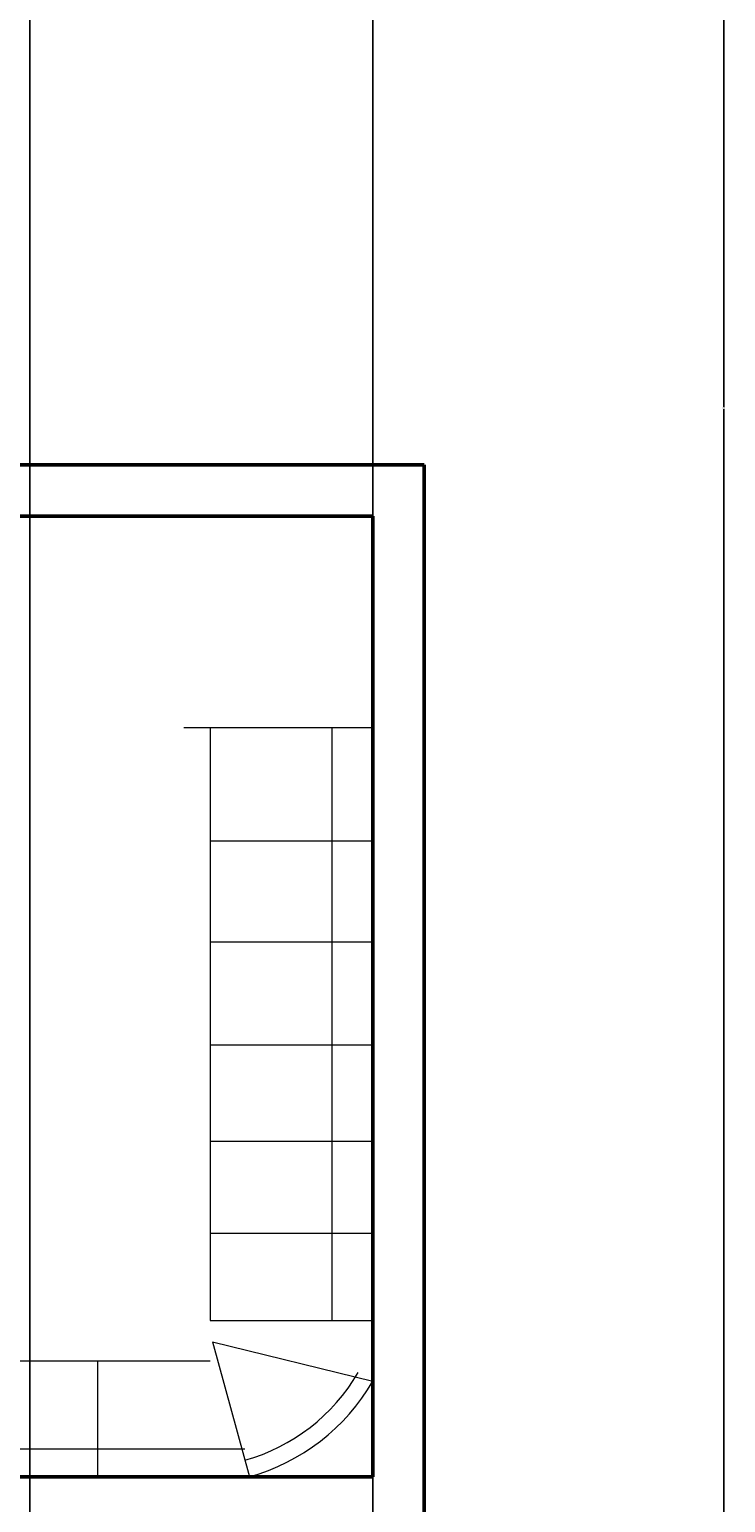
# Model space of a CAD drawing. Units: inches. Extents: x 5375 to 6084, y 16106 to 17259.
# Tile 26 of 32: x 5963 to 6084, y 16518 to 16776. Entities that reach past the tile are written whole.
import ezdxf

# ---------------------------------------------------------------- set-up
doc = ezdxf.new("R2010")
doc.units = ezdxf.units.IN
for name, color, linetype, lineweight in [('A-ANNO-DIMS', 2, 'Continuous', 18), ('FURNITURE', 3, 'Continuous', 18), ('WALL', 6, 'Continuous', 50)]:
    doc.layers.add(name, color=color, linetype=linetype, lineweight=lineweight)
doc.styles.get("Standard").update_dxf_attribs({"font": 'arial.ttf'})
doc.dimstyles.get("Standard").update_dxf_attribs({"dimtxt": 0.18, "dimasz": 0.18, "dimexe": 0.18, "dimexo": 0.0625, "dimgap": 0.09, "dimtad": 0, "dimtih": 1, "dimtoh": 1, "dimdec": 4, "dimzin": 0, "dimdsep": 46, "dimtxsty": 'Standard', "dimcen": 0.09, "dimadec": 0, "dimazin": 0, "dimtfac": 1, "dimtdec": 4, "dimtofl": 0, "dimtmove": 0, "dimatfit": 3, "dimfxl": 1, "dimtolj": 1, "dimtzin": 0, "dimarcsym": 0})

# ---------------------------------------------------------------- blocks, each defined once
blk = doc.blocks.new('*D31')
at = {"layer": 'A-ANNO-DIMS', "color": 0, "lineweight": -2, "transparency": 16777216}
for p, q in [((6031.68, 17206.58), (6084.2, 17206.58)), ((6084.02, 17206.4), (6084.02, 16709.66)), ((6084.02, 16212.56), (6084.02, 16709.3)), ((6031.68, 16212.38), (6084.2, 16212.38))]:
    blk.add_line(p, q, dxfattribs=at)
at = {"layer": 'A-ANNO-DIMS', "color": 0, "transparency": 16777216}
for points in [[(6083.99, 17206.4), (6084.05, 17206.4), (6084.02, 17206.58)], [(6083.99, 16212.56), (6084.05, 16212.56), (6084.02, 16212.38)]]:
    blk.add_solid(points, dxfattribs=at)
at = {"layer": 'Defpoints', "color": 0, "transparency": 16777216}
for p in [(6031.62, 17206.58), (6084.02, 17206.58), (6031.62, 16212.38)]:
    blk.add_point(p, dxfattribs=at)
at = {"layer": 'A-ANNO-DIMS', "color": 0, "transparency": 16777216, "insert": (6084.02, 16709.48), "char_height": 0.18, "attachment_point": 5}
blk.add_mtext('\\A1;994.2', dxfattribs=at)
blk = doc.blocks.new('*D48')
at = {"layer": 'A-ANNO-DIMS', "color": 0, "lineweight": -2, "transparency": 16777216}
for p, q in [((5962.62, 16411.64), (5962.62, 17259.16)), ((5962.8, 17258.98), (5992.4, 17258.98)), ((6022.44, 17258.98), (5992.84, 17258.98)), ((6022.62, 16411.64), (6022.62, 17259.16))]:
    blk.add_line(p, q, dxfattribs=at)
at = {"layer": 'A-ANNO-DIMS', "color": 0, "transparency": 16777216}
for points in [[(5962.8, 17259.01), (5962.8, 17258.95), (5962.62, 17258.98)], [(6022.44, 17259.01), (6022.44, 17258.95), (6022.62, 17258.98)]]:
    blk.add_solid(points, dxfattribs=at)
at = {"layer": 'Defpoints', "color": 0, "transparency": 16777216}
for p in [(6022.62, 17258.98), (5962.62, 16411.58), (6022.62, 16411.58)]:
    blk.add_point(p, dxfattribs=at)
at = {"layer": 'A-ANNO-DIMS', "color": 0, "transparency": 16777216, "insert": (5992.62, 17258.98), "char_height": 0.18, "attachment_point": 5}
blk.add_mtext('\\A1;60', dxfattribs=at)

msp = doc.modelspace()

# ---------------------------------------------------------------- linework, layer by layer
at = {"layer": 'FURNITURE'}
for p, q in [((5989.5486, 16653.6603), (6022.6199, 16653.6603)), ((5994.1715, 16653.6603), (5994.1715, 16549.933)), ((6015.4346, 16653.6603), (6015.4346, 16549.933)), ((6022.6199, 16653.6603), (6022.6199, 16539.3186)), ((5994.1715, 16633.797), (6022.6199, 16633.797)), ((5994.1715, 16616.1612), (6022.6199, 16616.1612)), ((5994.1715, 16598.1479), (6022.6199, 16598.1479)), ((5994.1715, 16581.2604), (6022.6199, 16581.2604)), ((5994.1715, 16565.2172), (6022.6199, 16565.2172)), ((5994.1715, 16549.933), (6022.6199, 16549.933)), ((5994.5739, 16546.2013), (6001.018, 16522.5793)), ((5994.5739, 16546.2013), (6022.6199, 16539.3186)), ((5859.7483, 16542.8395), (5994.1715, 16542.8395)), ((5974.4168, 16542.8395), (5974.4168, 16522.5793)), ((5859.7483, 16527.5002), (5974.4168, 16527.5002)), ((5974.4168, 16527.5002), (6000.2234, 16527.5002)), ((5859.7483, 16522.5793), (6001.018, 16522.5793))]:
    msp.add_line(p, q, dxfattribs=at)
for radius in [33.2909, 36.2909]:
    msp.add_arc((5991.2259, 16557.5242), radius, 285.653682, 329.890315, dxfattribs=at)
at = {"layer": 'WALL'}
for p, q in [((5950.6199, 16699.5793), (6031.6199, 16699.5793)), ((6031.6199, 16699.5793), (6031.6199, 16212.3785)), ((6031.6199, 16699.5793), (6031.6199, 16513.5793)), ((5800.6199, 16690.5793), (6022.6199, 16690.5793)), ((6022.6199, 16690.5793), (6022.6199, 16522.5793)), ((5800.6199, 16522.5793), (6022.6199, 16522.5793))]:
    msp.add_line(p, q, dxfattribs=at)

# ---------------------------------------------------------------- dimensions: what is measured, and where the dimension line sits
at = {"layer": 'A-ANNO-DIMS'}
dim = msp.add_linear_dim(base=(6022.6199, 17258.9793), p1=(5962.6199, 16411.5793), p2=(6022.6199, 16411.5793), dimstyle='Standard', override={"dimdec": 0, "dimlfac": 1, "dimrnd": 0, "dimzin": 0, "dimdsep": 46, "dimlunit": 2}, dxfattribs=at)
dim.commit()
dim.dimension.update_dxf_attribs({"geometry": '*D48', "text_midpoint": (5992.6199, 17258.9793)})
dim = msp.add_linear_dim(base=(6084.0199, 17206.5793), p1=(6031.6199, 16212.3785), p2=(6031.6199, 17206.5793), angle=90, dimstyle='Standard', override={"dimdec": 1, "dimlfac": 1, "dimrnd": 0, "dimzin": 0, "dimdsep": 46, "dimlunit": 2}, dxfattribs=at)
dim.commit()
dim.dimension.update_dxf_attribs({"geometry": '*D31', "text_midpoint": (6084.0199, 16709.4789)})

doc.saveas('drawing.dxf')
